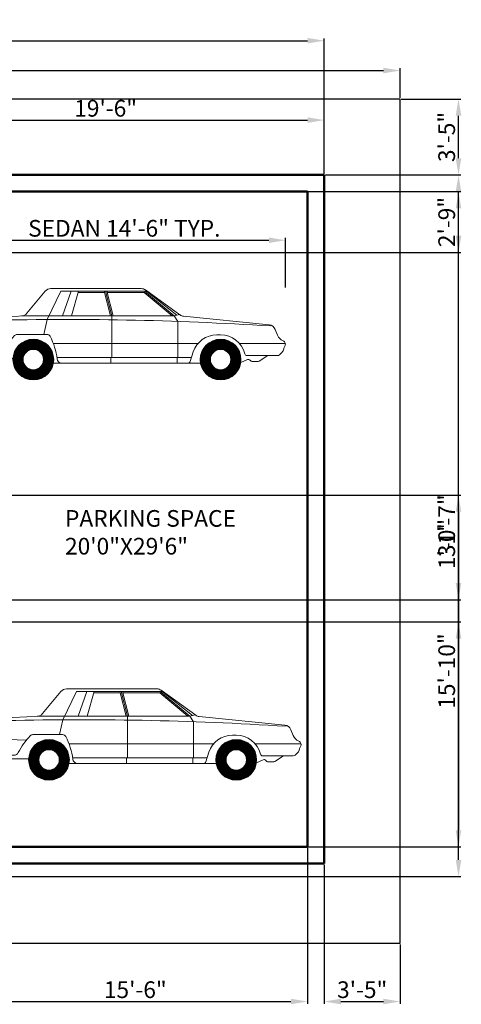
# Model space of a CAD drawing. Units: inches. Extents: x 2059616 to 2060276, y 889994 to 890582.
# Tile 4 of 4: x 2060037 to 2060276, y 890050 to 890582. Entities that reach past the tile are written whole.
import ezdxf

# ---------------------------------------------------------------- set-up
doc = ezdxf.new("R2010")
doc.units = ezdxf.units.IN
for name, color, linetype, lineweight in [('A-ANNO-DIMS', 2, 'Continuous', 18), ('A-AREA-IDEN', 7, 'Continuous', 25), ('A-SITE-VEHC', 8, 'Continuous', 18), ('A-WALL', 7, 'Continuous', 50), ('C-PROP', 7, 'Continuous', 25)]:
    doc.layers.add(name, color=color, linetype=linetype, lineweight=lineweight)
doc.styles.get("Standard").update_dxf_attribs({"font": 'arial.ttf'})
doc.dimstyles.new('ISO-25', dxfattribs={"dimtxt": 9, "dimasz": 9, "dimexe": 1.25, "dimexo": 0.625, "dimtad": 1, "dimdec": 1, "dimrnd": 9, "dimlunit": 3, "dimtxsty": 'Standard', "dimcen": 2.5, "dimadec": 0, "dimazin": 0, "dimtfac": 1, "dimtdec": 1, "dimtmove": 0, "dimatfit": 3, "dimfxl": 1, "dimarcsym": 0})

# ---------------------------------------------------------------- blocks, each defined once
blk = doc.blocks.new('*D1')
at = {"layer": 'A-ANNO-DIMS', "color": 0, "lineweight": -2, "transparency": 16777216}
for p, q in [((2059666.76, 890539.47), (2059666.76, 890555.48)), ((2059675.76, 890554.23), (2060233.76, 890554.23)), ((2060242.76, 890539.47), (2060242.76, 890555.48))]:
    blk.add_line(p, q, dxfattribs=at)
at = {"layer": 'A-ANNO-DIMS', "color": 0, "transparency": 16777216}
for points in [[(2059675.76, 890555.73), (2059675.76, 890552.73), (2059666.76, 890554.23)], [(2060233.76, 890555.73), (2060233.76, 890552.73), (2060242.76, 890554.23)]]:
    blk.add_solid(points, dxfattribs=at)
at = {"layer": 'Defpoints', "color": 0, "transparency": 16777216}
for p in [(2060242.76, 890554.23), (2059666.76, 890538.85), (2060242.76, 890538.85)]:
    blk.add_point(p, dxfattribs=at)
at = {"layer": 'A-ANNO-DIMS', "color": 0, "transparency": 16777216, "insert": (2059954.76, 890559.45), "char_height": 9, "attachment_point": 5}
blk.add_mtext("48'", dxfattribs=at)
blk = doc.blocks.new('Car - sedan  side')
for p, q in [((-139.53, 35.99), (-129.64, 47.91)), ((-128.57, 32.64), (-121.22, 48.02)), ((-77.81, 49.34), (-126.58, 49.34)), ((-74.7, 48.02), (-121.22, 48.02)), ((-120.32, 34.67), (-115.67, 48.02)), ((-115.4, 34.67), (-111.74, 48.02)), ((-94.41, 34.67), (-97.73, 48.02)), ((-93.72, 34.67), (-97.04, 48.02)), ((-93.03, 34.67), (-96.34, 48.02)), ((-60.02, 34.65), (-76.07, 48.02)), ((-56.87, 35.13), (-75.48, 48.59)), ((-58.54, 34.93), (-74.99, 48.02)), ((-97.55, 47.3), (-111.94, 47.3)), ((-76.26, 47.3), (-96.16, 47.3)), ((-61.08, 34.66), (-76.26, 47.3)), ((-140.23, 34.67), (-163.88, 33.56)), ((-62.28, 34.67), (-140.23, 34.67)), ((-130.39, 24.63), (-128.57, 32.64)), ((-93.72, 19.62), (-93.72, 34.67)), ((-62.28, 34.67), (-60.02, 34.65)), ((-60.02, 34.65), (-58.54, 34.93)), ((-57.97, 31.61), (-60.02, 34.65)), ((-57.21, 35.38), (-58.54, 34.93)), ((-54.93, 34.4), (-8.75, 29.8)), ((-170.93, 22.32), (-166.81, 31.56)), ((-164.57, 31.6), (-165.48, 30.35)), ((-57.97, 19.62), (-57.97, 31.61)), ((-4.21, 24.18), (-5.42, 27.27)), ((-148.26, 21.7), (-171.11, 22.33)), ((-128.78, 24.63), (-144.79, 24.63)), ((-36.97, 24.38), (-34.94, 24.38)), ((-174, 19.51), (-174, 18.91)), ((-160.12, 13.48), (-171.81, 16.16)), ((-47.2, 19.62), (-125.23, 19.62)), ((-93.72, 12.14), (-93.72, 19.62)), ((-57.97, 12.14), (-57.97, 19.62)), ((0, 19.62), (-24.7, 19.62)), ((-159.22, 12.14), (-161.08, 13.7)), ((-155.01, 13.48), (-160.12, 13.48)), ((-147.03, 11.6), (-157.73, 11.6)), ((-50.67, 12.14), (-123.32, 12.14)), ((-94.21, 9.03), (-94.21, 12.14)), ((-58.39, 9.03), (-58.39, 12.14)), ((-51.4, 9.89), (-49.69, 15.14)), ((-20.36, 11.06), (-24.06, 9.44)), ((-4.23, 13.19), (-20.72, 13.19)), ((-18.83, 10.42), (-19.11, 10.76)), ((-9.5, 13.19), (-14.1, 10.2)), ((-3.22, 13.59), (-1.77, 14.97)), ((-120.62, 9.03), (-125.23, 9.03)), ((-45.76, 9.03), (-120.62, 9.03)), ((-14.68, 10.03), (-18.01, 10.03))]:
    blk.add_line(p, q)
at = {"const_width": 5.49}
for points in [[(-127.8, 11, -1), (-144.3, 11, -1)], [(-26.69, 11, -1), (-43.19, 11, -1)]]:
    blk.add_lwpolyline(points, format="xyb", close=True, dxfattribs=at)
for centre, radius in [((-136.05, 11), 11), ((-34.94, 11), 11), ((-136.05, 11), 5.51), ((-34.94, 11), 5.51)]:
    blk.add_circle(centre, radius)
for centre, radius, start, end in [((-126.58, 45.38), 3.97, 90, 140.3029), ((-77.81, 45.38), 3.97, 54.135, 90), ((-163.72, 30.18), 3.38, 92.6827, 155.9736), ((-163.62, 30.91), 1.17, 91.491, 143.9553), ((-118.51, -1702.12), 1734.79, 86.34698, 91.49105), ((-142.58, 38.53), 3.97, 272.6827, 320.3029), ((-54.54, 38.35), 3.97, 234.135, 264.3123), ((-9.15, 25.82), 4, 21.3107, 84.3123), ((-171.18, 19.51), 2.82, 88.4193, 180), ((-118.09, -2.78), 38.85, 136.3964, 152.9097), ((-144.79, 22.64), 1.98, 90, 136.3964), ((-128.78, 22.64), 1.98, 28.1371, 90), ((-157.14, 7.48), 34.14, 6.5135, 28.1371), ((-36.97, 11), 13.38, 90, 161.9732), ((-34.94, 11), 13.38, 13.5864, 90), ((0.9, 26.18), 5.49, 201.3107, 247.7048), ((-171.18, 18.91), 2.82, 180, 257.0905), ((-3.82, 17.12), 2.96, 313.7173, 352.3839), ((-1.92, 19.3), 1.94, 325.3744, 67.7048), ((2.46, 16.28), 3.37, 145.3744, 172.3839), ((-157.73, 13.93), 2.32, 230.1291, 270), ((-155.01, 16.1), 2.62, 270, 332.9097), ((-120.62, 11.65), 2.62, 186.5135, 270), ((-20.72, 14.43), 1.24, 193.5864, 270), ((-19.93, 10.09), 1.06, 39.301, 113.7159), ((-4.23, 14.65), 1.46, 270, 313.7173), ((-52.58, 10.27), 1.24, 270, 341.9732), ((-18.01, 11.09), 1.06, 219.301, 270), ((-14.68, 11.09), 1.06, 270, 303.047)]:
    blk.add_arc(centre, radius, start, end)
blk = doc.blocks.new('*D13')
at = {"layer": 'A-ANNO-DIMS', "color": 0, "lineweight": -2, "transparency": 16777216}
for p, q in [((2059965.76, 890498.47), (2059965.76, 890528.71)), ((2059974.76, 890527.46), (2060192.76, 890527.46)), ((2060201.76, 890498.47), (2060201.76, 890528.71))]:
    blk.add_line(p, q, dxfattribs=at)
at = {"layer": 'A-ANNO-DIMS', "color": 0, "transparency": 16777216}
for points in [[(2059974.76, 890528.96), (2059974.76, 890525.96), (2059965.76, 890527.46)], [(2060192.76, 890528.96), (2060192.76, 890525.96), (2060201.76, 890527.46)]]:
    blk.add_solid(points, dxfattribs=at)
at = {"layer": 'Defpoints', "color": 0, "transparency": 16777216}
for p in [(2060201.76, 890527.46), (2059965.76, 890497.85), (2060201.76, 890497.85)]:
    blk.add_point(p, dxfattribs=at)
at = {"layer": 'A-ANNO-DIMS', "color": 0, "transparency": 16777216, "insert": (2060083.76, 890532.68), "char_height": 9, "attachment_point": 5}
blk.add_mtext('19\'-6"', dxfattribs=at)
blk = doc.blocks.new('*D20')
at = {"layer": 'A-ANNO-DIMS', "color": 0, "lineweight": -2, "transparency": 16777216}
for p, q in [((2060006.77, 890437.07), (2060006.77, 890463.82)), ((2060015.77, 890462.57), (2060171.88, 890462.57)), ((2060180.88, 890437.07), (2060180.88, 890463.82))]:
    blk.add_line(p, q, dxfattribs=at)
at = {"layer": 'A-ANNO-DIMS', "color": 0, "transparency": 16777216}
for points in [[(2060015.77, 890464.07), (2060015.77, 890461.07), (2060006.77, 890462.57)], [(2060171.88, 890464.07), (2060171.88, 890461.07), (2060180.88, 890462.57)]]:
    blk.add_solid(points, dxfattribs=at)
at = {"layer": 'Defpoints', "color": 0, "transparency": 16777216}
for p in [(2060180.88, 890462.57), (2060006.77, 890436.45), (2060180.88, 890436.45)]:
    blk.add_point(p, dxfattribs=at)
at = {"layer": 'A-ANNO-DIMS', "color": 0, "transparency": 16777216, "insert": (2060093.82, 890467.84), "char_height": 9, "attachment_point": 5}
blk.add_mtext('SEDAN 14\'-6" TYP.', dxfattribs=at)
blk = doc.blocks.new('*D38')
at = {"layer": 'A-ANNO-DIMS', "color": 0, "lineweight": -2, "transparency": 16777216}
for p, q in [((2059689.91, 890369.47), (2059689.91, 890571.6)), ((2059698.91, 890570.35), (2060192.76, 890570.35)), ((2060201.76, 890498.47), (2060201.76, 890571.6))]:
    blk.add_line(p, q, dxfattribs=at)
at = {"layer": 'A-ANNO-DIMS', "color": 0, "transparency": 16777216}
for points in [[(2059698.91, 890571.85), (2059698.91, 890568.85), (2059689.91, 890570.35)], [(2060192.76, 890571.85), (2060192.76, 890568.85), (2060201.76, 890570.35)]]:
    blk.add_solid(points, dxfattribs=at)
at = {"layer": 'Defpoints', "color": 0, "transparency": 16777216}
for p in [(2060201.76, 890570.35), (2060201.76, 890497.85), (2059689.91, 890368.85)]:
    blk.add_point(p, dxfattribs=at)
at = {"layer": 'A-ANNO-DIMS', "color": 0, "transparency": 16777216, "insert": (2059945.84, 890575.57), "char_height": 9, "attachment_point": 5}
blk.add_mtext('42\'-8"', dxfattribs=at)
blk = doc.blocks.new('*D39')
at = {"layer": 'A-ANNO-DIMS', "color": 0, "lineweight": -2, "transparency": 16777216}
for p, q in [((2060202.39, 890497.85), (2060275.51, 890497.85)), ((2060274.26, 890127.85), (2060274.26, 890488.85)), ((2059926.39, 890118.85), (2060275.51, 890118.85))]:
    blk.add_line(p, q, dxfattribs=at)
at = {"layer": 'A-ANNO-DIMS', "color": 0, "transparency": 16777216}
for points in [[(2060272.76, 890488.85), (2060275.76, 890488.85), (2060274.26, 890497.85)], [(2060272.76, 890127.85), (2060275.76, 890127.85), (2060274.26, 890118.85)]]:
    blk.add_solid(points, dxfattribs=at)
at = {"layer": 'Defpoints', "color": 0, "transparency": 16777216}
for p in [(2060201.76, 890497.85), (2060274.26, 890497.85), (2059925.76, 890118.85)]:
    blk.add_point(p, dxfattribs=at)
at = {"layer": 'A-ANNO-DIMS', "color": 0, "transparency": 16777216, "insert": (2060269.04, 890308.35), "char_height": 9, "attachment_point": 5, "rotation": 90}
blk.add_mtext('31\'-7"', dxfattribs=at)
blk = doc.blocks.new('*D43')
at = {"layer": 'A-ANNO-DIMS', "color": 0, "lineweight": -2, "transparency": 16777216}
for p, q in [((2060243.39, 890538.85), (2060275.51, 890538.85)), ((2060274.26, 890506.85), (2060274.26, 890529.85)), ((2060202.39, 890497.85), (2060275.51, 890497.85))]:
    blk.add_line(p, q, dxfattribs=at)
at = {"layer": 'A-ANNO-DIMS', "color": 0, "transparency": 16777216}
for points in [[(2060272.76, 890529.85), (2060275.76, 890529.85), (2060274.26, 890538.85)], [(2060272.76, 890506.85), (2060275.76, 890506.85), (2060274.26, 890497.85)]]:
    blk.add_solid(points, dxfattribs=at)
at = {"layer": 'Defpoints', "color": 0, "transparency": 16777216}
for p in [(2060242.76, 890538.85), (2060274.26, 890538.85), (2060201.76, 890497.85)]:
    blk.add_point(p, dxfattribs=at)
at = {"layer": 'A-ANNO-DIMS', "color": 0, "transparency": 16777216, "insert": (2060269.04, 890518.35), "char_height": 9, "attachment_point": 5, "rotation": 90}
blk.add_mtext('3\'-5"', dxfattribs=at)
blk = doc.blocks.new('*D44')
at = {"layer": 'A-ANNO-DIMS', "color": 0, "lineweight": -2, "transparency": 16777216}
for p, q in [((2060201.76, 890125.22), (2060201.76, 890050.1)), ((2060242.76, 890082.22), (2060242.76, 890050.1)), ((2060210.76, 890051.35), (2060233.76, 890051.35))]:
    blk.add_line(p, q, dxfattribs=at)
at = {"layer": 'A-ANNO-DIMS', "color": 0, "transparency": 16777216}
for points in [[(2060210.76, 890052.85), (2060210.76, 890049.85), (2060201.76, 890051.35)], [(2060233.76, 890052.85), (2060233.76, 890049.85), (2060242.76, 890051.35)]]:
    blk.add_solid(points, dxfattribs=at)
at = {"layer": 'Defpoints', "color": 0, "transparency": 16777216}
for p in [(2060201.76, 890125.85), (2060242.76, 890082.85), (2060242.76, 890051.35)]:
    blk.add_point(p, dxfattribs=at)
at = {"layer": 'A-ANNO-DIMS', "color": 0, "transparency": 16777216, "insert": (2060222.26, 890056.57), "char_height": 9, "attachment_point": 5}
blk.add_mtext('3\'-5"', dxfattribs=at)
blk = doc.blocks.new('*D53')
at = {"layer": 'A-ANNO-DIMS', "color": 0, "lineweight": -2, "transparency": 16777216}
for p, q in [((2059975.39, 890488.85), (2060275.51, 890488.85)), ((2060274.26, 890464.97), (2060274.26, 890479.85)), ((2059975.39, 890455.97), (2060275.51, 890455.97))]:
    blk.add_line(p, q, dxfattribs=at)
at = {"layer": 'A-ANNO-DIMS', "color": 0, "transparency": 16777216}
for points in [[(2060272.76, 890479.85), (2060275.76, 890479.85), (2060274.26, 890488.85)], [(2060272.76, 890464.97), (2060275.76, 890464.97), (2060274.26, 890455.97)]]:
    blk.add_solid(points, dxfattribs=at)
at = {"layer": 'Defpoints', "color": 0, "transparency": 16777216}
for p in [(2059974.76, 890488.85), (2060274.26, 890488.85), (2059974.76, 890455.97)]:
    blk.add_point(p, dxfattribs=at)
at = {"layer": 'A-ANNO-DIMS', "color": 0, "transparency": 16777216, "insert": (2060269.04, 890472.41), "char_height": 9, "attachment_point": 5, "rotation": 90}
blk.add_mtext('2\'-9"', dxfattribs=at)
blk = doc.blocks.new('*D55')
at = {"layer": 'A-ANNO-DIMS', "color": 0, "lineweight": -2, "transparency": 16777216}
for p, q in [((2060007.39, 890324.89), (2060275.51, 890324.89)), ((2060274.26, 890315.89), (2060274.26, 890143.85)), ((2060007.39, 890134.85), (2060275.51, 890134.85))]:
    blk.add_line(p, q, dxfattribs=at)
at = {"layer": 'A-ANNO-DIMS', "color": 0, "transparency": 16777216}
for points in [[(2060272.76, 890315.89), (2060275.76, 890315.89), (2060274.26, 890324.89)], [(2060272.76, 890143.85), (2060275.76, 890143.85), (2060274.26, 890134.85)]]:
    blk.add_solid(points, dxfattribs=at)
at = {"layer": 'Defpoints', "color": 0, "transparency": 16777216}
for p in [(2060006.76, 890324.89), (2060006.76, 890134.85), (2060274.26, 890134.85)]:
    blk.add_point(p, dxfattribs=at)
at = {"layer": 'A-ANNO-DIMS', "color": 0, "transparency": 16777216, "insert": (2060269.04, 890229.87), "char_height": 9, "attachment_point": 5, "rotation": 90}
blk.add_mtext('15\'-10"', dxfattribs=at)
blk = doc.blocks.new('*D56')
at = {"layer": 'A-ANNO-DIMS', "color": 0, "lineweight": -2, "transparency": 16777216}
for p, q in [((2060006.76, 890134.22), (2060006.76, 890050.1)), ((2060192.76, 890134.22), (2060192.76, 890050.1)), ((2060015.76, 890051.35), (2060183.76, 890051.35))]:
    blk.add_line(p, q, dxfattribs=at)
at = {"layer": 'A-ANNO-DIMS', "color": 0, "transparency": 16777216}
for points in [[(2060015.76, 890052.85), (2060015.76, 890049.85), (2060006.76, 890051.35)], [(2060183.76, 890052.85), (2060183.76, 890049.85), (2060192.76, 890051.35)]]:
    blk.add_solid(points, dxfattribs=at)
at = {"layer": 'Defpoints', "color": 0, "transparency": 16777216}
for p in [(2060006.76, 890134.85), (2060192.76, 890134.85), (2060192.76, 890051.35)]:
    blk.add_point(p, dxfattribs=at)
at = {"layer": 'A-ANNO-DIMS', "color": 0, "transparency": 16777216, "insert": (2060099.76, 890056.57), "char_height": 9, "attachment_point": 5}
blk.add_mtext('15\'-6"', dxfattribs=at)
blk = doc.blocks.new('*D59')
at = {"layer": 'A-ANNO-DIMS', "color": 0, "lineweight": -2, "transparency": 16777216}
for p, q in [((2060274.26, 890277.39), (2060274.26, 890310.71)), ((2059926.39, 890268.39), (2060275.51, 890268.39)), ((2060274.26, 890256.39), (2060274.26, 890268.39)), ((2059926.39, 890256.39), (2060275.51, 890256.39)), ((2060274.26, 890247.39), (2060274.26, 890238.39))]:
    blk.add_line(p, q, dxfattribs=at)
at = {"layer": 'A-ANNO-DIMS', "color": 0, "transparency": 16777216}
for points in [[(2060272.76, 890277.39), (2060275.76, 890277.39), (2060274.26, 890268.39)], [(2060272.76, 890247.39), (2060275.76, 890247.39), (2060274.26, 890256.39)]]:
    blk.add_solid(points, dxfattribs=at)
at = {"layer": 'Defpoints', "color": 0, "transparency": 16777216}
for p in [(2059925.76, 890268.39), (2060274.26, 890268.39), (2059925.76, 890256.39)]:
    blk.add_point(p, dxfattribs=at)
at = {"layer": 'A-ANNO-DIMS', "color": 0, "transparency": 16777216, "insert": (2060269.04, 890298.55), "char_height": 9, "attachment_point": 5, "rotation": 90}
blk.add_mtext('1\'-0"', dxfattribs=at)

msp = doc.modelspace()

# ---------------------------------------------------------------- linework, layer by layer
at = {"layer": 'A-WALL'}
for p, q in [((2060201.76, 890497.85), (2059707.76, 890497.85)), ((2060201.76, 890125.85), (2060201.76, 890497.85)), ((2060192.76, 890488.85), (2059974.76, 890488.85)), ((2060192.76, 890134.85), (2060192.76, 890488.85)), ((2060192.76, 890134.85), (2060006.76, 890134.85)), ((2060192.76, 890125.85), (2059997.76, 890125.85)), ((2060192.76, 890125.85), (2060201.76, 890125.85))]:
    msp.add_line(p, q, dxfattribs=at)
at = {"layer": 'C-PROP'}
for p, q in [((2060242.76, 890538.85), (2059666.76, 890538.85)), ((2060242.76, 890082.85), (2060242.76, 890538.85)), ((2059666.76, 890082.85), (2060242.76, 890082.85))]:
    msp.add_line(p, q, dxfattribs=at)

# ---------------------------------------------------------------- block references
at = {"layer": 'A-SITE-VEHC'}
for p in [(2060180.77, 890387.1), (2060189.23, 890170.88)]:
    msp.add_blockref('Car - sedan  side', p, dxfattribs=at)

# ---------------------------------------------------------------- texts
at = {"layer": 'A-AREA-IDEN', "insert": (2060061.83, 890316.81), "char_height": 9, "attachment_point": 1}
msp.add_mtext_dynamic_manual_height_columns('PARKING SPACE\\P20\'0"X29\'6"', width=120.7712, gutter_width=12.5, heights=[0], dxfattribs=at)

# ---------------------------------------------------------------- dimensions: what is measured, and where the dimension line sits
at = {"layer": 'A-ANNO-DIMS'}
for base, p1, p2, override, picture, middle in [((2060201.7635, 890570.3463), (2059689.9147, 890368.8463), (2060201.7635, 890497.8463), {"dimdec": 1, "dimlfac": 1, "dimrnd": 0, "dimzin": 1, "dimdsep": 46, "dimlunit": 4, "dimfrac": 2}, '*D38', (2059945.8391, 890575.5665)), ((2060242.76, 890554.23), (2059666.76, 890538.85), (2060242.76, 890538.85), {"dimclrd": 0, "dimclre": 0, "dimclrt": 0}, '*D1', (2059954.76, 890559.45)), ((2060201.76, 890527.46), (2059965.76, 890497.85), (2060201.76, 890497.85), {"dimclrd": 0, "dimclre": 0, "dimclrt": 0}, '*D13', (2060083.76, 890532.68)), ((2060192.76, 890051.35), (2060006.76, 890134.85), (2060192.76, 890134.85), {"dimdec": 1, "dimlfac": 1, "dimrnd": 0, "dimzin": 1, "dimdsep": 46, "dimlunit": 4, "dimfrac": 2}, '*D56', (2060099.76, 890056.57)), ((2060242.76, 890051.35), (2060201.76, 890125.85), (2060242.76, 890082.85), {"dimdec": 1, "dimlfac": 1, "dimrnd": 0, "dimzin": 1, "dimdsep": 46, "dimlunit": 4, "dimfrac": 2}, '*D44', (2060222.26, 890056.57))]:
    dim = msp.add_linear_dim(base=base, p1=p1, p2=p2, dimstyle='ISO-25', override=override, dxfattribs=at)
    dim.commit()
    dim.dimension.update_dxf_attribs({"geometry": picture, "text_midpoint": middle})
for base, p1, p2, picture, middle in [((2060274.26, 890538.85), (2060201.76, 890497.85), (2060242.76, 890538.85), '*D43', (2060269.04, 890518.35)), ((2060274.26, 890497.85), (2059925.76, 890118.85), (2060201.76, 890497.85), '*D39', (2060269.04, 890308.35)), ((2060274.26, 890488.85), (2059974.76, 890455.97), (2059974.76, 890488.85), '*D53', (2060269.04, 890472.41)), ((2060274.26, 890134.85), (2060006.76, 890324.89), (2060006.76, 890134.85), '*D55', (2060269.04, 890229.87)), ((2060274.26, 890268.39), (2059925.76, 890256.39), (2059925.76, 890268.39), '*D59', (2060269.04, 890298.55))]:
    dim = msp.add_linear_dim(base=base, p1=p1, p2=p2, angle=90, dimstyle='ISO-25', override={"dimdec": 1, "dimlfac": 1, "dimrnd": 0, "dimzin": 1, "dimdsep": 46, "dimlunit": 4, "dimfrac": 2}, dxfattribs=at)
    dim.commit()
    dim.dimension.update_dxf_attribs({"geometry": picture, "text_midpoint": middle})
dim = msp.add_linear_dim(base=(2060180.88, 890462.57), p1=(2060006.77, 890436.45), p2=(2060180.88, 890436.45), text='SEDAN <> TYP.', dimstyle='ISO-25', override={"dimdec": 1, "dimlfac": 1, "dimrnd": 0, "dimzin": 1, "dimdsep": 46, "dimlunit": 4, "dimfrac": 2}, dxfattribs=at)
dim.commit()
dim.dimension.update_dxf_attribs({"geometry": '*D20', "text_midpoint": (2060093.82, 890467.84)})

doc.saveas('drawing.dxf')
